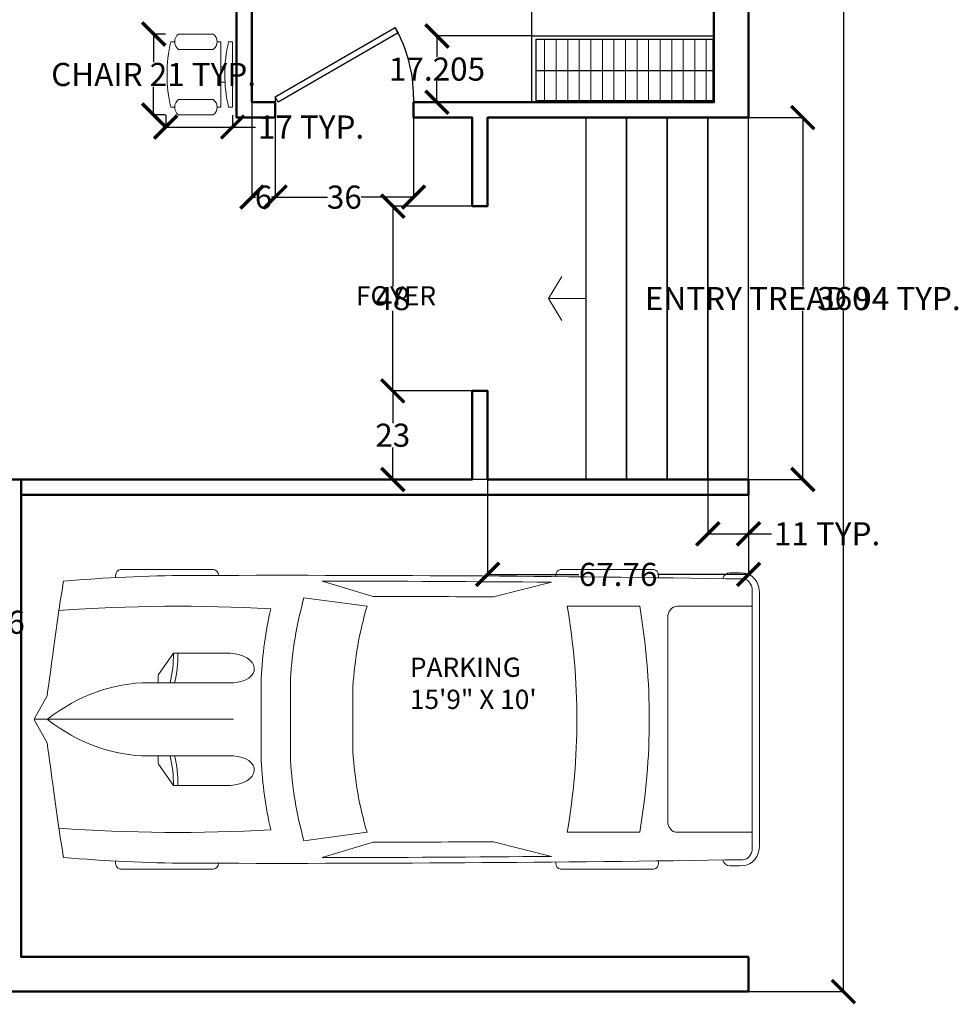
# Model space of a CAD drawing. Units: inches. Extents: x 9 to 573, y -373 to 44.
# Tile 4 of 5: x 329 to 573, y -348 to -92. Entities that reach past the tile are written whole.
import ezdxf

# ---------------------------------------------------------------- set-up
doc = ezdxf.new("R2010")
doc.units = ezdxf.units.IN
doc.header["$MEASUREMENT"] = 0
for name, color, linetype, lineweight in [('A-ANNO-DIMS', 2, 'Continuous', 18), ('A-ANNO-SYMB', 3, 'Continuous', 18), ('A-AREA-IDEN', 7, 'Continuous', 25), ('A-DOOR', 4, 'Continuous', 25), ('A-FLOR-CASE', 8, 'Continuous', 25), ('A-FLOR-CASE-PATT', 252, 'Continuous', 13), ('A-FLOR-STRS', 7, 'Continuous', 25), ('A-FURN', 8, 'Continuous', 18), ('A-SITE-VEHC', 8, 'Continuous', 13), ('A-WALL', 7, 'Continuous', 50)]:
    doc.layers.add(name, color=color, linetype=linetype, lineweight=lineweight)
doc.styles.get("Standard").update_dxf_attribs({"font": 'arial.ttf'})
doc.dimstyles.get("Standard").update_dxf_attribs({"dimtxt": 6, "dimasz": 6, "dimexe": 0.18, "dimexo": 0.0625, "dimgap": 0.09, "dimtad": 0, "dimtih": 1, "dimtoh": 1, "dimdec": 0, "dimzin": 0, "dimdsep": 46, "dimlunit": 4, "dimtxsty": 'Standard', "dimblk": 'ARCHTICK', "dimcen": 0.09, "dimadec": 0, "dimazin": 0, "dimtfac": 1, "dimtdec": 0, "dimtofl": 0, "dimtmove": 0, "dimatfit": 3, "dimldrblk": 'ARCHTICK', "dimfxl": 1, "dimtolj": 1, "dimtzin": 0, "dimarcsym": 0})

# ---------------------------------------------------------------- blocks, each defined once
blk = doc.blocks.new('*U3')
for p, q in [((0, 0), (0, -6)), ((40, 0), (40, -6))]:
    blk.add_line(p, q)
blk.add_lwpolyline([(0, 0), (34.64, 20), (35.52, 18.48), (0.88, -1.52)], close=True)
blk.add_arc((0, 0), 40, 0, 30)
blk = doc.blocks.new('Chair - Desk')
for p, q in [((-8.5, 0), (-8.5, -1)), ((-8.5, 0), (8.5, 0)), ((8.5, 0), (8.5, -1)), ((-2, -3), (-2, -1.9355)), ((2, -1.9576), (2, -3)), ((-10.5, -5), (-10.5, -14)), ((-8.5, -3), (-8.5, -4)), ((-8.5, -3), (8.5, -3)), ((-6.5, -14), (-6.5, -5)), ((6.5, -5), (6.5, -14)), ((8.5, -3), (8.5, -4)), ((10.5, -14), (10.5, -5)), ((-8.5, -15), (-8.5, -16)), ((8.5, -15), (8.5, -16))]:
    blk.add_line(p, q)
for centre, radius, start, end in [((0, 34.625), 36.625, 256.5803, 283.4197), ((-8.5, -6.5), 2.5, 36.8699, 143.1301), ((8.5, -6.5), 2.5, 36.8699, 143.1301), ((-8.5, -12.5), 2.5, 216.8699, 323.1301), ((8.5, -12.5), 2.5, 216.8699, 323.1301), ((0, 19.625), 36.625, 256.5803, 283.4197)]:
    blk.add_arc(centre, radius, start, end)
blk = doc.blocks.new('*U27')
for p, q in [((46.55, 38.89), (22.35, 38.89)), ((136.7, 38.89), (160.9, 38.89)), ((21.1, 37.41), (21.1, 36.83)), ((47.8, 37.39), (47.8, 37.41)), ((87.99, 31.87), (74.76, 35.92)), ((135.45, 37.07), (135.45, 37.41)), ((162.15, 37.41), (162.15, 36.77)), ((134.31, 35.6), (119.29, 31.78)), ((186.47, -33.5), (186.47, 33.5)), ((70.03, 31.54), (86.41, 29.35)), ((188.4, -32.76), (188.4, 32.76)), ((138.42, 29.35), (157.25, 29.35)), ((186.47, 29.35), (167.01, 29.35)), ((164.52, 26.39), (164.52, -26.39)), ((32.27, 11.63), (36.13, 17.17)), ((36.13, 17.17), (50.94, 17.17)), ((32.12, 9.51), (32.12, 11.15)), ((58.92, -10.77), (58.92, 10.77)), ((66.55, -10.53), (66.55, 10.53)), ((186.47, -10.53), (186.47, 10.53)), ((29.77, 9.51), (51.68, 9.51)), ((82.74, 8.5), (82.74, -8.5)), ((3.27, 6.13), (0.1, 0.41)), ((0, 0), (51.68, 0)), ((0.1, -0.41), (3.27, -6.13)), ((29.77, -9.51), (51.68, -9.51)), ((32.12, -9.51), (32.12, -11.15)), ((32.27, -11.63), (36.13, -17.17)), ((36.13, -17.17), (50.94, -17.17)), ((86.41, -29.35), (70.03, -31.54)), ((157.25, -29.35), (138.42, -29.35)), ((167.01, -29.35), (186.47, -29.35)), ((87.99, -31.87), (74.76, -35.92)), ((134.31, -35.6), (119.29, -31.78)), ((21.1, -37.41), (21.1, -36.83)), ((47.8, -37.39), (47.8, -37.41)), ((135.45, -37.07), (135.45, -37.41)), ((162.15, -37.41), (162.15, -36.77)), ((46.55, -38.89), (22.35, -38.89)), ((136.7, -38.89), (160.9, -38.89))]:
    blk.add_line(p, q)
for centre, major_axis, ratio, start_param, end_param in [((22.35, 37.41), (0, -1.48), 0.842304, 3.141593, 4.712389), ((46.55, 37.41), (0, 1.48), 0.842304, -1.570796, 0), ((136.7, 37.41), (0, -1.48), 0.842304, 3.141593, 4.712389), ((160.9, 37.41), (0, 1.48), 0.842304, -1.570796, 0), ((266.03, -27.52), (0, 313.31), 0.842304, 1.367076, 1.39176), ((41.19, -490.86), (0, 528.23), 0.842304, 0.00281, 0.075598), ((64.48, -10555.62), (0, 10593.03), 0.842304, -0.013397, 0.002797), ((64.48, -10555.62), (0, -10591.55), 0.842304, 3.133765, 3.140441), ((180.63, 35.84), (0, 2.22), 0.842304, -0.013017, 1.249894), ((64.48, -10556.36), (0, 10595.31), 0.842304, -0.013397, -0.013017), ((183.98, 33.5), (0, -2.96), 0.842304, 1.570796, 3.128196), ((183.98, 32.76), (0, -5.25), 0.842304, 1.570796, 3.128196), ((135.29, 5.39), (0, 81.77), 0.842304, 1.245306, 1.50788), ((95.79, -3666.35), (0, -3698.24), 0.842304, 3.134049, 3.144098), ((259.18, -27.52), (0, -305.3), 0.842304, 4.528606, 4.561838), ((37.47, -593.96), (0, -623.33), 0.842304, 3.096046, 3.200911), ((134.4, 5.39), (0, -89.78), 0.842304, 4.449482, 4.652344), ((149.6, 2.8), (0, -79.58), 0.842304, 4.372215, 4.640744), ((17.08, 0), (0, 147.02), 0.842304, 4.511394, 4.913384), ((35.91, 0), (0, 147.02), 0.842304, 4.511394, 4.913384), ((167.01, 26.39), (0, 2.96), 0.842304, 0, 1.570796), ((-204.49, 52.4), (0, -250.96), 0.842304, 1.385369, 1.434372), ((13.04, 17.01), (0, 27.42), 0.842304, 4.435146, 4.718221), ((14.2, 17.01), (0, 27.42), 0.842304, 4.435146, 4.718221), ((50.79, 13.34), (6.34, -0.36), 0.603834, -1.395552, 1.581315), ((32.75, 11.15), (0, 0.74), 0.842304, 0.879714, 1.570796), ((29.77, -46.66), (0, 56.17), 0.842304, 0, 0.590319), ((0.62, 0), (0, -0.74), 0.842304, 4.131459, 5.293319), ((29.77, 46.66), (0, 56.17), 0.842304, 2.551274, 3.141593), ((-204.49, -52.4), (0, 250.96), 0.842304, -1.434372, -1.385369), ((13.04, -17.01), (0, -27.42), 0.842304, 1.564964, 1.848039), ((14.2, -17.01), (0, -27.42), 0.842304, 1.564964, 1.848039), ((149.6, -2.8), (0, -79.58), 0.842304, -1.499151, -1.230623), ((32.75, -11.15), (0, -0.74), 0.842304, 4.712389, 5.403472), ((134.4, -5.39), (0, -89.78), 0.842304, -1.510751, -1.307889), ((135.29, -5.39), (0, -81.77), 0.842304, -1.50788, -1.245306), ((259.18, 27.52), (0, 305.3), 0.842304, 1.721348, 1.754579), ((167.01, -26.39), (0, -2.96), 0.842304, 4.712389, 6.283185), ((266.03, 27.52), (0, 313.31), 0.842304, 1.749832, 1.774517), ((37.47, 593.96), (0, -623.33), 0.842304, -0.059319, 0.045547), ((95.79, 3666.35), (0, -3698.24), 0.842304, -0.002505, 0.007544), ((183.98, -32.76), (0, -5.25), 0.842304, 0.013397, 1.570796), ((64.48, 10555.62), (0, -10591.55), 0.842304, 0.001152, 0.007828), ((183.98, -33.5), (0, 2.96), 0.842304, 3.15499, 4.712389), ((41.19, 490.86), (0, -528.23), 0.842304, -0.075598, -0.00281), ((22.35, -37.41), (0, 1.48), 0.842304, 1.570796, 3.141593), ((64.48, 10555.62), (0, 10593.03), 0.842304, 3.138796, 3.15499), ((46.55, -37.41), (0, -1.48), 0.842304, 0, 1.570796), ((136.7, -37.41), (0, -1.48), 0.842304, -1.570796, 0), ((160.9, -37.41), (0, 1.48), 0.842304, 3.141593, 4.712389), ((180.63, -35.84), (0, -2.22), 0.842304, -1.249894, 0.013017), ((64.48, 10556.36), (0, 10595.31), 0.842304, 3.15461, 3.15499)]:
    blk.add_ellipse(centre, major_axis=major_axis, ratio=ratio, start_param=start_param, end_param=end_param)
at = {"extrusion": (0, 0, -1)}
blk.add_ellipse((50.79, -13.34), major_axis=(6.34, 0.36), ratio=0.603834, start_param=-1.395552, end_param=1.581315, dxfattribs=at)
blk = doc.blocks.new('ENTRY-STAIR-TREAD')
blk.add_lwpolyline([(10.56, 94), (0, 94), (0, 0), (10.56, 0)], close=True)
blk = doc.blocks.new('_ArchTick')
at = {"color": 0, "linetype": 'ByBlock', "const_width": 0.15}
blk.add_lwpolyline([(-0.5, -0.5), (0.5, 0.5)], dxfattribs=at)
blk = doc.blocks.new('*D30')
at = {"layer": 'A-ANNO-DIMS', "color": 0, "lineweight": -2, "transparency": 16777216}
for p, q in [((193.52, -70), (193.52, -82.12)), ((273.52, -70), (273.52, -82.12)), ((193.52, -81.94), (273.52, -81.94)), ((273.52, -81.94), (279.52, -81.94))]:
    blk.add_line(p, q, dxfattribs=at)
at = {"layer": 'Defpoints', "color": 0, "transparency": 16777216}
for p in [(193.52, -69.94), (273.52, -69.94), (273.52, -81.94)]:
    blk.add_point(p, dxfattribs=at)
at = {"layer": 'A-ANNO-DIMS', "color": 0, "lineweight": -2, "transparency": 16777216, "xscale": 6, "yscale": 6, "zscale": 6, "rotation": 180}
blk.add_blockref('_ArchTick', (193.52, -81.94), dxfattribs=at)
at = {"layer": 'A-ANNO-DIMS', "color": 0, "lineweight": -2, "transparency": 16777216, "xscale": 6, "yscale": 6, "zscale": 6}
blk.add_blockref('_ArchTick', (273.52, -81.94), dxfattribs=at)
at = {"layer": 'A-ANNO-DIMS', "color": 0, "transparency": 16777216, "insert": (320.05, -81.94), "char_height": 6, "attachment_point": 5}
blk.add_mtext('\\A1;QUEEN BED 80 TYP.', dxfattribs=at)
blk = doc.blocks.new('*D34')
at = {"layer": 'A-ANNO-DIMS', "color": 0, "lineweight": -2, "transparency": 16777216}
for p, q in [((518.58, -117.2), (532.8, -117.2)), ((532.62, -117.2), (532.62, -161.04)), ((532.62, -211.2), (532.62, -167.35)), ((518.58, -211.2), (532.8, -211.2))]:
    blk.add_line(p, q, dxfattribs=at)
at = {"layer": 'Defpoints', "color": 0, "transparency": 16777216}
for p in [(518.52, -117.2), (532.62, -117.2), (518.52, -211.2)]:
    blk.add_point(p, dxfattribs=at)
at = {"layer": 'A-ANNO-DIMS', "color": 0, "lineweight": -2, "transparency": 16777216, "xscale": 6, "yscale": 6, "zscale": 6}
for p, rotation in [((532.62, -117.2), 90), ((532.62, -211.2), 270)]:
    blk.add_blockref('_ArchTick', p, dxfattribs=dict(at, rotation=rotation))
at = {"layer": 'A-ANNO-DIMS', "color": 0, "transparency": 16777216, "insert": (532.62, -164.2), "char_height": 6, "attachment_point": 5}
blk.add_mtext('\\A1;ENTRY TREAD 94 TYP.', dxfattribs=at)
blk = doc.blocks.new('*D35')
at = {"layer": 'A-ANNO-DIMS', "color": 0, "lineweight": -2, "transparency": 16777216}
for p, q in [((507.96, -211.26), (507.96, -225.48)), ((518.52, -211.26), (518.52, -225.48)), ((507.96, -225.3), (518.52, -225.3)), ((518.52, -225.3), (524.52, -225.3))]:
    blk.add_line(p, q, dxfattribs=at)
at = {"layer": 'Defpoints', "color": 0, "transparency": 16777216}
for p in [(507.96, -211.2), (518.52, -211.2), (518.52, -225.3)]:
    blk.add_point(p, dxfattribs=at)
at = {"layer": 'A-ANNO-DIMS', "color": 0, "lineweight": -2, "transparency": 16777216, "xscale": 6, "yscale": 6, "zscale": 6, "rotation": 180}
blk.add_blockref('_ArchTick', (507.96, -225.3), dxfattribs=at)
at = {"layer": 'A-ANNO-DIMS', "color": 0, "lineweight": -2, "transparency": 16777216, "xscale": 6, "yscale": 6, "zscale": 6}
blk.add_blockref('_ArchTick', (518.52, -225.3), dxfattribs=at)
at = {"layer": 'A-ANNO-DIMS', "color": 0, "transparency": 16777216, "insert": (538.93, -225.3), "char_height": 6, "attachment_point": 5}
blk.add_mtext('\\A1;11 TYP.', dxfattribs=at)
blk = doc.blocks.new('*D42')
at = {"layer": 'A-ANNO-DIMS', "color": 0, "lineweight": -2, "transparency": 16777216}
for p, q in [((367.06, -95.49), (363.79, -95.49)), ((363.97, -95.49), (363.97, -102.8)), ((363.97, -116.49), (363.97, -109.18)), ((367.06, -116.49), (363.79, -116.49))]:
    blk.add_line(p, q, dxfattribs=at)
at = {"layer": 'Defpoints', "color": 0, "transparency": 16777216}
for p in [(367.12, -95.49), (363.97, -116.49), (367.12, -116.49)]:
    blk.add_point(p, dxfattribs=at)
at = {"layer": 'A-ANNO-DIMS', "color": 0, "lineweight": -2, "transparency": 16777216, "xscale": 6, "yscale": 6, "zscale": 6}
for p, rotation in [((363.97, -95.49), 90), ((363.97, -116.49), 270)]:
    blk.add_blockref('_ArchTick', p, dxfattribs=dict(at, rotation=rotation))
at = {"layer": 'A-ANNO-DIMS', "color": 0, "transparency": 16777216, "insert": (363.97, -105.99), "char_height": 6, "attachment_point": 5}
blk.add_mtext('\\A1;CHAIR 21 TYP.', dxfattribs=at)
blk = doc.blocks.new('*D43')
at = {"layer": 'A-ANNO-DIMS', "color": 0, "lineweight": -2, "transparency": 16777216}
for p, q in [((367.12, -116.55), (367.12, -119.82)), ((384.45, -116.55), (384.45, -119.82)), ((367.12, -119.64), (384.45, -119.64)), ((384.45, -119.64), (390.45, -119.64))]:
    blk.add_line(p, q, dxfattribs=at)
at = {"layer": 'Defpoints', "color": 0, "transparency": 16777216}
for p in [(367.12, -116.49), (384.45, -116.49), (384.45, -119.64)]:
    blk.add_point(p, dxfattribs=at)
at = {"layer": 'A-ANNO-DIMS', "color": 0, "lineweight": -2, "transparency": 16777216, "xscale": 6, "yscale": 6, "zscale": 6, "rotation": 180}
blk.add_blockref('_ArchTick', (367.12, -119.64), dxfattribs=at)
at = {"layer": 'A-ANNO-DIMS', "color": 0, "lineweight": -2, "transparency": 16777216, "xscale": 6, "yscale": 6, "zscale": 6}
blk.add_blockref('_ArchTick', (384.45, -119.64), dxfattribs=at)
at = {"layer": 'A-ANNO-DIMS', "color": 0, "transparency": 16777216, "insert": (404.86, -119.64), "char_height": 6, "attachment_point": 5}
blk.add_mtext('\\A1;17 TYP.', dxfattribs=at)
blk = doc.blocks.new('*D52')
at = {"layer": 'A-ANNO-DIMS', "color": 0, "lineweight": -2, "transparency": 16777216}
for p, q in [((304.13, -230.28), (298.62, -230.28)), ((298.8, -230.28), (298.79, -245.08)), ((298.77, -266.28), (298.78, -251.48)), ((304.11, -266.28), (298.59, -266.28))]:
    blk.add_line(p, q, dxfattribs=at)
at = {"layer": 'Defpoints', "color": 0, "transparency": 16777216}
for p in [(304.2, -230.28), (298.77, -266.28), (304.17, -266.28)]:
    blk.add_point(p, dxfattribs=at)
at = {"layer": 'A-ANNO-DIMS', "color": 0, "lineweight": -2, "transparency": 16777216, "xscale": 6, "yscale": 6, "zscale": 6}
for p, rotation in [((298.8, -230.28), 89.96776293761982), ((298.77, -266.28), 269.9677629376198)]:
    blk.add_blockref('_ArchTick', p, dxfattribs=dict(at, rotation=rotation))
at = {"layer": 'A-ANNO-DIMS', "color": 0, "transparency": 16777216, "insert": (298.78, -248.28), "char_height": 6, "attachment_point": 5}
blk.add_mtext('\\A1;DOUBLE SINK 36', dxfattribs=at)
blk = doc.blocks.new('*D59')
at = {"layer": 'A-ANNO-DIMS', "color": 0, "lineweight": -2, "transparency": 16777216}
for p, q in [((518.58, 15.8), (543.35, 15.8)), ((543.17, 15.8), (543.17, -161.04)), ((543.17, -344.2), (543.17, -167.35)), ((518.58, -344.2), (543.35, -344.2))]:
    blk.add_line(p, q, dxfattribs=at)
at = {"layer": 'Defpoints', "color": 0, "transparency": 16777216}
for p in [(518.52, 15.8), (518.52, -344.2), (543.17, -344.2)]:
    blk.add_point(p, dxfattribs=at)
at = {"layer": 'A-ANNO-DIMS', "color": 0, "lineweight": -2, "transparency": 16777216, "xscale": 6, "yscale": 6, "zscale": 6}
for p, rotation in [((543.17, 15.8), 90), ((543.17, -344.2), 270)]:
    blk.add_blockref('_ArchTick', p, dxfattribs=dict(at, rotation=rotation))
at = {"layer": 'A-ANNO-DIMS', "color": 0, "transparency": 16777216, "insert": (543.17, -164.2), "char_height": 6, "attachment_point": 5}
blk.add_mtext('\\A1;360', dxfattribs=at)
blk = doc.blocks.new('*D65')
at = {"layer": 'A-ANNO-DIMS', "color": 0, "lineweight": -2, "transparency": 16777216}
for p, q in [((450.69, -140.2), (425.92, -140.2)), ((426.1, -140.2), (426.1, -161.04)), ((426.1, -188.2), (426.1, -167.35)), ((450.69, -188.2), (425.92, -188.2))]:
    blk.add_line(p, q, dxfattribs=at)
at = {"layer": 'Defpoints', "color": 0, "transparency": 16777216}
for p in [(426.1, -140.2), (450.75, -140.2), (450.75, -188.2)]:
    blk.add_point(p, dxfattribs=at)
at = {"layer": 'A-ANNO-DIMS', "color": 0, "lineweight": -2, "transparency": 16777216, "xscale": 6, "yscale": 6, "zscale": 6}
for p, rotation in [((426.1, -140.2), 90), ((426.1, -188.2), 270)]:
    blk.add_blockref('_ArchTick', p, dxfattribs=dict(at, rotation=rotation))
at = {"layer": 'A-ANNO-DIMS', "color": 0, "transparency": 16777216, "insert": (426.1, -164.2), "char_height": 6, "attachment_point": 5}
blk.add_mtext('\\A1;48', dxfattribs=at)
blk = doc.blocks.new('*D66')
at = {"layer": 'A-ANNO-DIMS', "color": 0, "lineweight": -2, "transparency": 16777216}
for p, q in [((450.75, -211.26), (450.75, -236.03)), ((518.52, -211.26), (518.52, -236.03)), ((450.75, -235.85), (474.41, -235.85)), ((518.52, -235.85), (494.86, -235.85))]:
    blk.add_line(p, q, dxfattribs=at)
at = {"layer": 'Defpoints', "color": 0, "transparency": 16777216}
for p in [(450.75, -211.2), (518.52, -211.2), (450.75, -235.85)]:
    blk.add_point(p, dxfattribs=at)
at = {"layer": 'A-ANNO-DIMS', "color": 0, "lineweight": -2, "transparency": 16777216, "xscale": 6, "yscale": 6, "zscale": 6, "rotation": 180}
blk.add_blockref('_ArchTick', (450.75, -235.85), dxfattribs=at)
at = {"layer": 'A-ANNO-DIMS', "color": 0, "lineweight": -2, "transparency": 16777216, "xscale": 6, "yscale": 6, "zscale": 6}
blk.add_blockref('_ArchTick', (518.52, -235.85), dxfattribs=at)
at = {"layer": 'A-ANNO-DIMS', "color": 0, "transparency": 16777216, "insert": (484.64, -235.85), "char_height": 6, "attachment_point": 5}
blk.add_mtext('\\A1;67.76', dxfattribs=at)
blk = doc.blocks.new('*D67')
at = {"layer": 'A-ANNO-DIMS', "color": 0, "lineweight": -2, "transparency": 16777216}
for p, q in [((450.69, -188.2), (425.92, -188.2)), ((426.1, -188.2), (426.1, -196.54)), ((426.1, -211.2), (426.1, -202.85)), ((450.69, -211.2), (425.92, -211.2))]:
    blk.add_line(p, q, dxfattribs=at)
at = {"layer": 'Defpoints', "color": 0, "transparency": 16777216}
for p in [(426.1, -188.2), (450.75, -188.2), (450.75, -211.2)]:
    blk.add_point(p, dxfattribs=at)
at = {"layer": 'A-ANNO-DIMS', "color": 0, "lineweight": -2, "transparency": 16777216, "xscale": 6, "yscale": 6, "zscale": 6}
for p, rotation in [((426.1, -188.2), 90), ((426.1, -211.2), 270)]:
    blk.add_blockref('_ArchTick', p, dxfattribs=dict(at, rotation=rotation))
at = {"layer": 'A-ANNO-DIMS', "color": 0, "transparency": 16777216, "insert": (426.1, -199.7), "char_height": 6, "attachment_point": 5}
blk.add_mtext('\\A1;23', dxfattribs=at)
blk = doc.blocks.new('*D84')
at = {"layer": 'A-ANNO-DIMS', "color": 0, "lineweight": -2, "transparency": 16777216}
for p, q in [((389.52, -113.26), (389.52, -138.03)), ((395.52, -113.26), (395.52, -138.03)), ((389.52, -137.85), (390.45, -137.85)), ((395.52, -137.85), (394.59, -137.85))]:
    blk.add_line(p, q, dxfattribs=at)
at = {"layer": 'Defpoints', "color": 0, "transparency": 16777216}
for p in [(389.52, -113.2), (395.52, -113.2), (389.52, -137.85)]:
    blk.add_point(p, dxfattribs=at)
at = {"layer": 'A-ANNO-DIMS', "color": 0, "lineweight": -2, "transparency": 16777216, "xscale": 6, "yscale": 6, "zscale": 6, "rotation": 180}
blk.add_blockref('_ArchTick', (389.52, -137.85), dxfattribs=at)
at = {"layer": 'A-ANNO-DIMS', "color": 0, "lineweight": -2, "transparency": 16777216, "xscale": 6, "yscale": 6, "zscale": 6}
blk.add_blockref('_ArchTick', (395.52, -137.85), dxfattribs=at)
at = {"layer": 'A-ANNO-DIMS', "color": 0, "transparency": 16777216, "insert": (392.52, -137.85), "char_height": 6, "attachment_point": 5}
blk.add_mtext('\\A1;6', dxfattribs=at)
blk = doc.blocks.new('*D85')
at = {"layer": 'A-ANNO-DIMS', "color": 0, "lineweight": -2, "transparency": 16777216}
for p, q in [((395.52, -113.26), (395.52, -138.03)), ((431.52, -113.26), (431.52, -138.03)), ((395.52, -137.85), (409.13, -137.85)), ((431.52, -137.85), (417.9, -137.85))]:
    blk.add_line(p, q, dxfattribs=at)
at = {"layer": 'Defpoints', "color": 0, "transparency": 16777216}
for p in [(395.52, -113.2), (431.52, -113.2), (395.52, -137.85)]:
    blk.add_point(p, dxfattribs=at)
at = {"layer": 'A-ANNO-DIMS', "color": 0, "lineweight": -2, "transparency": 16777216, "xscale": 6, "yscale": 6, "zscale": 6, "rotation": 180}
blk.add_blockref('_ArchTick', (395.52, -137.85), dxfattribs=at)
at = {"layer": 'A-ANNO-DIMS', "color": 0, "lineweight": -2, "transparency": 16777216, "xscale": 6, "yscale": 6, "zscale": 6}
blk.add_blockref('_ArchTick', (431.52, -137.85), dxfattribs=at)
at = {"layer": 'A-ANNO-DIMS', "color": 0, "transparency": 16777216, "insert": (413.52, -137.85), "char_height": 6, "attachment_point": 5}
blk.add_mtext('\\A1;36', dxfattribs=at)
blk = doc.blocks.new('*D91')
at = {"layer": 'A-ANNO-DIMS', "color": 0, "lineweight": -2, "transparency": 16777216}
for p, q in [((462.17, -95.99), (437.41, -95.99)), ((437.59, -95.99), (437.59, -101.44)), ((437.59, -113.2), (437.59, -107.75)), ((462.17, -113.2), (437.41, -113.2))]:
    blk.add_line(p, q, dxfattribs=at)
at = {"layer": 'Defpoints', "color": 0, "transparency": 16777216}
for p in [(437.59, -95.99), (462.24, -95.99), (462.24, -113.2)]:
    blk.add_point(p, dxfattribs=at)
at = {"layer": 'A-ANNO-DIMS', "color": 0, "lineweight": -2, "transparency": 16777216, "xscale": 6, "yscale": 6, "zscale": 6}
for p, rotation in [((437.59, -95.99), 90), ((437.59, -113.2), 270)]:
    blk.add_blockref('_ArchTick', p, dxfattribs=dict(at, rotation=rotation))
at = {"layer": 'A-ANNO-DIMS', "color": 0, "transparency": 16777216, "insert": (437.59, -104.59), "char_height": 6, "attachment_point": 5}
blk.add_mtext('\\A1;17.205', dxfattribs=at)
blk = doc.blocks.new('*D92')
at = {"layer": 'A-ANNO-DIMS', "color": 0, "lineweight": -2, "transparency": 16777216}
for p, q in [((462.24, -95.93), (462.24, -71.16)), ((462.24, -71.34), (475.54, -71.34)), ((509.52, -71.34), (496.22, -71.34)), ((509.52, -95.93), (509.52, -71.16))]:
    blk.add_line(p, q, dxfattribs=at)
at = {"layer": 'Defpoints', "color": 0, "transparency": 16777216}
for p in [(509.52, -71.34), (462.24, -95.99), (509.52, -95.99)]:
    blk.add_point(p, dxfattribs=at)
at = {"layer": 'A-ANNO-DIMS', "color": 0, "lineweight": -2, "transparency": 16777216, "xscale": 6, "yscale": 6, "zscale": 6, "rotation": 180}
blk.add_blockref('_ArchTick', (462.24, -71.34), dxfattribs=at)
at = {"layer": 'A-ANNO-DIMS', "color": 0, "lineweight": -2, "transparency": 16777216, "xscale": 6, "yscale": 6, "zscale": 6}
blk.add_blockref('_ArchTick', (509.52, -71.34), dxfattribs=at)
at = {"layer": 'A-ANNO-DIMS', "color": 0, "transparency": 16777216, "insert": (485.88, -71.34), "char_height": 6, "attachment_point": 5}
blk.add_mtext('\\A1;47.28', dxfattribs=at)

msp = doc.modelspace()

# ---------------------------------------------------------------- hatches: boundary and pattern name
at = {"layer": 'A-FLOR-CASE-PATT'}
h = msp.add_hatch(dxfattribs=at)
h.set_pattern_fill('ANSI31', color=256, scale=24, angle=45, style=0)
h.set_pattern_definition([(90, (-716.4455, -458.4915), (-3, 0), [])])
h.paths.add_polyline_path([(463.274, -112.7864), (509.274, -112.7864), (509.274, -96.7864), (463.274, -96.7864)])

# ---------------------------------------------------------------- linework, layer by layer
at = {"layer": 'A-ANNO-SYMB'}
msp.add_line((476.281, -164.1966), (466.5545, -164.1966), dxfattribs=at)
msp.add_lwpolyline([(470.0545, -158.4915), (466.5545, -164.1966), (470.0545, -169.9017)], dxfattribs=at)
at = {"layer": 'A-FLOR-CASE'}
for p, q in [((462.2364, -113.1966), (462.2364, -95.9915)), ((462.2364, -95.9915), (509.5169, -95.9915)), ((463.274, -96.7864), (509.274, -96.7864)), ((463.274, -96.7864), (463.274, -112.7864)), ((509.274, -96.7864), (509.274, -112.7864)), ((463.274, -104.9915), (509.274, -104.9915)), ((463.274, -112.7864), (509.274, -112.7864))]:
    msp.add_line(p, q, dxfattribs=at)
at = {"layer": 'A-WALL'}
for p, q in [((518.5169, -211.1966), (450.7536, -211.1966)), ((518.5169, -215.1966), (518.5169, -211.1966)), ((509.5169, -215.1966), (518.5169, -215.1966))]:
    msp.add_line(p, q, dxfattribs=at)
for points in [[(329.5169, -215.1966), (329.5169, -335.1966), (509.5169, -335.1966), (518.5169, -335.1966), (518.5169, -344.1966), (38.5169, -344.1966), (38.5169, 15.8034), (518.5169, 15.8034), (518.5169, -117.1966), (450.7536, -117.1966), (450.7536, -140.1966), (446.7536, -140.1966), (446.7536, -117.1966), (431.5169, -117.1966), (431.5169, -113.1966), (509.5169, -113.1966), (509.5169, 6.8034), (389.5169, 6.8034), (389.5169, -113.1966), (395.5169, -113.1966), (395.5169, -117.1966), (385.5169, -117.1966), (385.5169, 6.8034), (325.5169, 6.8034)], [(450.7536, -211.1966), (450.7536, -188.1966), (446.7536, -188.1966), (446.7536, -211.1966), (298.5169, -211.1966), (298.5169, -215.1966), (325.5169, -215.1966), (325.5169, -335.1966), (241.5169, -335.1966), (241.5169, -215.1966), (268.5169, -215.1966), (268.5169, -211.1966), (241.5169, -211.1966), (237.5169, -211.1966), (237.5169, -215.1966), (237.5169, -335.1966), (195.5169, -335.1966), (195.5169, -215.1966)], [(509.5169, -215.1966), (329.5169, -215.1966), (329.5169, -211.1966)]]:
    msp.add_lwpolyline(points, dxfattribs=at)

# ---------------------------------------------------------------- block references
at = {"layer": 'A-DOOR', "xscale": 0.9, "yscale": 0.9, "zscale": 0.9}
msp.add_blockref('*U3', (395.5169, -111.7966), dxfattribs=at)
at = {"layer": 'A-FLOR-STRS'}
for p in [(476.2811, -211.197), (486.8401, -211.197), (497.399, -211.197), (507.958, -211.197)]:
    msp.add_blockref('ENTRY-STAIR-TREAD', p, dxfattribs=at)
at = {"layer": 'A-FURN', "rotation": 270}
msp.add_blockref('Chair - Desk', (384.4523, -105.9915), dxfattribs=at)
at = {"layer": 'A-SITE-VEHC'}
msp.add_blockref('*U27', (333.0044, -273.4915), dxfattribs=at)

# ---------------------------------------------------------------- texts
at = {"layer": 'A-AREA-IDEN', "char_height": 5, "attachment_point": 1}
for s, width, insert in [('FOYER', 113.199185, (416.5545, -160.9915)), ('PARKING \\P15\'9" X 10\'', 174.489033, (430.5545, -257.4672))]:
    msp.add_mtext_dynamic_manual_height_columns(s, width=width, gutter_width=1, heights=[0], dxfattribs=dict(at, insert=insert))

# ---------------------------------------------------------------- dimensions: what is measured, and where the dimension line sits
at = {"layer": 'A-ANNO-DIMS'}
for base, p1, p2, angle, override, picture, middle in [((543.1669, -344.1966), (518.5169, 15.8034), (518.5169, -344.1966), 270, {"dimdec": 0, "dimlfac": 1, "dimrnd": 0, "dimzin": 0, "dimdsep": 46, "dimlunit": 2}, '*D59', (543.1669, -164.1966)), ((437.5864, -95.9915), (462.2364, -113.1966), (462.2364, -95.9915), 90, {"dimdec": 3, "dimlfac": 1, "dimrnd": 0, "dimzin": 0, "dimdsep": 46, "dimlunit": 2}, '*D91', (437.5864, -104.5941)), ((389.5169, -137.8466), (395.5169, -113.1966), (389.5169, -113.1966), 180, {"dimdec": 0, "dimlfac": 1, "dimrnd": 0, "dimzin": 0, "dimdsep": 46, "dimlunit": 2}, '*D84', (392.5169, -137.8466)), ((395.5169, -137.8466), (431.5169, -113.1966), (395.5169, -113.1966), 180, {"dimdec": 0, "dimlfac": 1, "dimrnd": 0, "dimzin": 0, "dimdsep": 46, "dimlunit": 2}, '*D85', (413.5169, -137.8466)), ((426.1036, -140.1966), (450.7536, -188.1966), (450.7536, -140.1966), 90, {"dimdec": 0, "dimlfac": 1, "dimrnd": 0, "dimzin": 0, "dimdsep": 46, "dimlunit": 2}, '*D65', (426.1036, -164.1966)), ((426.1036, -188.1966), (450.7536, -211.1966), (450.7536, -188.1966), 90, {"dimdec": 0, "dimlfac": 1, "dimrnd": 0, "dimzin": 0, "dimdsep": 46, "dimlunit": 2}, '*D67', (426.1036, -199.6966)), ((450.7536, -235.8466), (518.5169, -211.1966), (450.7536, -211.1966), 180, {"dimdec": 2, "dimlfac": 1, "dimrnd": 0, "dimzin": 0, "dimdsep": 46, "dimlunit": 2}, '*D66', (484.6353, -235.8466))]:
    dim = msp.add_linear_dim(base=base, p1=p1, p2=p2, angle=angle, dimstyle='Standard', override=override, dxfattribs=at)
    dim.commit()
    dim.dimension.update_dxf_attribs({"geometry": picture, "text_midpoint": middle})
for base, p1, p2, text, picture, middle in [((273.5169, -81.9382), (193.5168, -69.9382), (273.5169, -69.9382), 'QUEEN BED <> TYP.', '*D30', (320.0537, -81.9382)), ((384.4523, -119.6415), (367.1189, -116.4915), (384.4523, -116.4915), '<> TYP.', '*D43', (404.8629, -119.6415)), ((518.5169, -225.2966), (507.9579, -211.1966), (518.5169, -211.1966), '<> TYP.', '*D35', (538.9275, -225.2966))]:
    dim = msp.add_linear_dim(base=base, p1=p1, p2=p2, text=text, dimstyle='Standard', override={"dimdec": 0, "dimlfac": 1, "dimrnd": 0, "dimzin": 0, "dimdsep": 46, "dimlunit": 2}, dxfattribs=at)
    dim.commit()
    dim.dimension.update_dxf_attribs({"geometry": picture, "text_midpoint": middle})
dim = msp.add_linear_dim(base=(509.5169, -71.3415), p1=(462.2364, -95.9915), p2=(509.5169, -95.9915), dimstyle='Standard', override={"dimdec": 2, "dimlfac": 1, "dimrnd": 0, "dimzin": 0, "dimdsep": 46, "dimlunit": 2}, dxfattribs=at)
dim.commit()
dim.dimension.update_dxf_attribs({"geometry": '*D92', "text_midpoint": (485.8766, -71.3415)})
for base, p1, p2, angle, text, picture, middle in [((363.9689, -116.4915), (367.1189, -95.4915), (367.1189, -116.4915), 270, 'CHAIR <> TYP.', '*D42', (363.9689, -105.9915)), ((532.6169, -117.1966), (518.5169, -211.1966), (518.5169, -117.1966), 90, 'ENTRY TREAD <> TYP.', '*D34', (532.6169, -164.1966)), ((298.7749, -266.2786), (304.1951, -230.2817), (304.1749, -266.2817), 269.967763, 'DOUBLE SINK <>', '*D52', (298.785, -248.2786))]:
    dim = msp.add_linear_dim(base=base, p1=p1, p2=p2, angle=angle, text=text, dimstyle='Standard', override={"dimdec": 0, "dimlfac": 1, "dimrnd": 0, "dimzin": 0, "dimdsep": 46, "dimlunit": 2}, dxfattribs=at)
    dim.commit()
    dim.dimension.update_dxf_attribs({"geometry": picture, "text_midpoint": middle})

doc.saveas('drawing.dxf')
